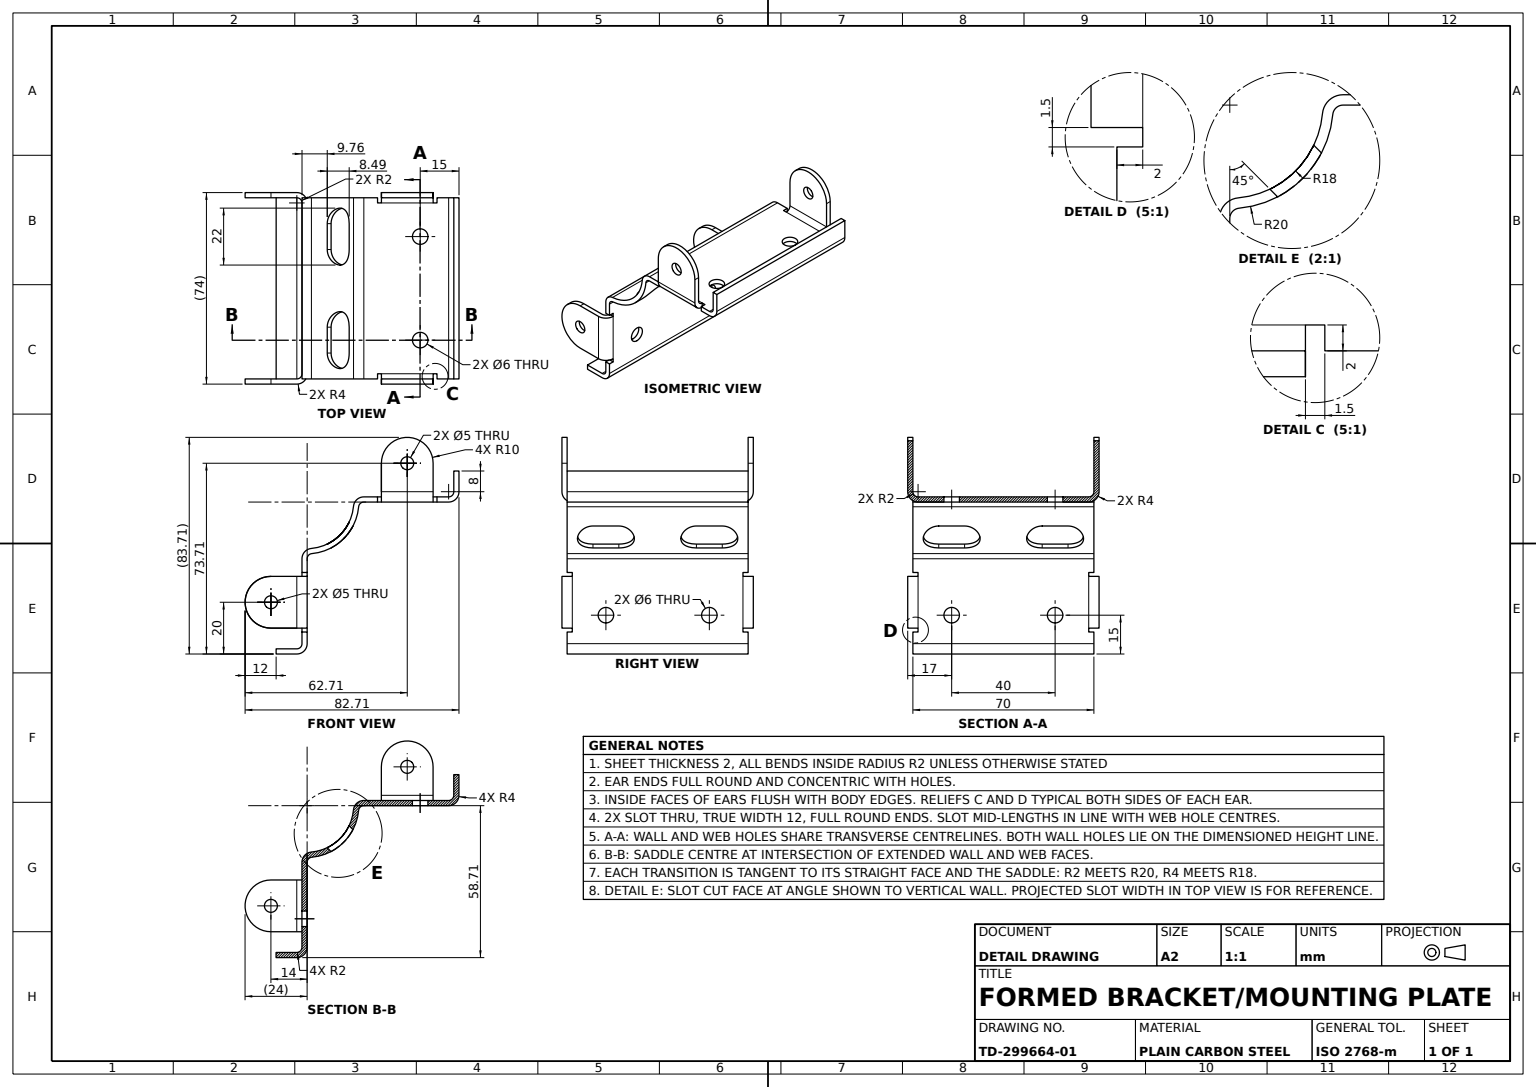
SolidWorks part; units mm, degrees
material "Plain Carbon Steel"
ref_plane "Front Plane" through (0, 0, 0) normal (0, 0, 1) x (1, 0, 0)
ref_plane "Top Plane" through (0, 0, 0) normal (0, 1, 0) x (1, 0, 0)
ref_plane "Right Plane" through (0, 0, 0) normal (1, 0, 0) x (0, 0, -1)
sketch "Saddle Profile Sketch" plane through (0, 0, 0) normal (0, 0, 1) x (1, 0, 0)
  line L0 (-15.4919, -15.4919) -> (-38.6863, -38.6863)
  line L1 (15.4919, -15.4919) -> (38.6863, -38.6863)
  line L9 (-44.3431, -38.6863) -> (-50, -33.0294)
  line L10 (42.9289, -37.2721) -> (48.5858, -31.6152)
  line L11 (44.3431, -38.6863) -> (50, -33.0294)
  line L12 (-50, -50) -> (-50, -50.1773)
  line L13 (-41.5147, -41.5147) -> (-15.4919, -15.4919)
  line L14 (16.9061, -14.0777) -> (40.1005, -37.2721)
  line L15 (-16.9061, -14.0777) -> (-40.1005, -37.2721)
  line L16 (41.5147, -41.5147) -> (15.4919, -15.4919)
  line L17 (-42.9289, -37.2721) -> (-48.5858, -31.6152)
  line L18 (-50, -33.0294) -> (-48.5858, -31.6152)
  line L19 (50, -33.0294) -> (48.5858, -31.6152)
  arc A0 (-12.7979, -15.3692) -> (12.7979, -15.3692) centre (0, 0) ccw
  arc A1 (38.6863, -38.6863) -> (44.3431, -38.6863) centre (41.5147, -35.8579) ccw
  arc A2 (-44.3431, -38.6863) -> (-38.6863, -38.6863) centre (-41.5147, -35.8579) ccw
  arc A3 (12.7979, -15.3692) -> (15.4919, -15.4919) centre (14.0777, -16.9061) cw
  arc A4 (-12.7979, -15.3692) -> (-15.4919, -15.4919) centre (-14.0777, -16.9061) ccw
  arc A5 (40.1005, -37.2721) -> (42.9289, -37.2721) centre (41.5147, -35.8579) ccw
  arc A6 (11.5181, -13.8323) -> (16.9061, -14.0777) centre (14.0777, -16.9061) cw
  arc A7 (-11.5181, -13.8323) -> (11.5181, -13.8323) centre (0, 0) ccw
  arc A8 (-11.5181, -13.8323) -> (-16.9061, -14.0777) centre (-14.0777, -16.9061) ccw
  arc A9 (-42.9289, -37.2721) -> (-40.1005, -37.2721) centre (-41.5147, -35.8579) ccw
  point P8 (0, 0)
  dimension "D1" = 40
  dimension "D5" = 4
  dimension "D6" = 2
  dimension "D2" = 45
  dimension "D3" = 45
  dimension "D4" = 8.4853
  dimension "D7" = 50
  dimension "D8" = 50
  dimension "D9" = 23.1944
  dimension "D10" = 23.1944
  dimension "D11" = 8
  dimension "D13" = 0.1773
  dimension "D14" = 50
  dimension "D15" = 50
  dimension "D12" = 2
extrude "Saddle Body 70mm" add sketch "Saddle Profile Sketch" along normal blind 70 contours A9 L17 L18 L9 A2 L0 A4 A0 A3 L1 A1 L11 L19 L10 A5 L14 A6 A7 A8 L15
sketch "Flange Notches Sketch" plane through (0, 0, 0) normal (0, 1, 0) x (1, 0, 0)
  line L0 (-6, -10) -> (-6, -20)
  line L1 (6, -10) -> (6, -20)
  line L2 (16.9061, 0) -> (40.1005, 0) construction
  line L3 (-6, -50) -> (-6, -60)
  line L4 (6, -50) -> (6, -60)
  line L6 (16.9061, -70) -> (40.1005, -70) construction
  line L8 (11.5181, -70) -> (11.5181, 0) construction
  arc A0 (6, -10) -> (-6, -10) centre (0, -10) ccw
  arc A1 (-6, -20) -> (6, -20) centre (0, -20) ccw
  arc A2 (6, -50) -> (-6, -50) centre (0, -50) ccw
  arc A3 (-6, -60) -> (6, -60) centre (0, -60) ccw
  point P1 (6, -15)
  point P5 (6, -55)
  dimension "D1" = 10
  dimension "D2" = 6
  dimension "D3" = 15
  dimension "D5" = 6
  dimension "D4" = 10
  dimension "D6" = 15
  dimension "D7" = 10
  dimension "D8" = 11.5181
extrude "Flange Notches" cut sketch "Flange Notches Sketch" against normal blind 70
sketch "Flange Holes A Sketch" plane through (1.4142, 1.4142, 0) normal (0.7071, 0.7071, 0) x (0, 0, -1)
  line L0 (-70, -21.9089) -> (-70, -54.7107) construction
  line L1 (0, -21.9089) -> (0, -54.7107) construction
  line L3 (-70, -58.7107) -> (0, -58.7107) construction
  circle A0 centre (-55, -43.7107) radius 3
  circle A1 centre (-15, -43.7107) radius 3
  dimension "D1" = 6
  dimension "D2" = 6
  dimension "D3" = 15
  dimension "D4" = 15
  dimension "D5" = 40
  dimension "D6" = 15
extrude "Flange Holes A Ø6" cut sketch "Flange Holes A Sketch" against normal blind 70
sketch "Flange Holes B Sketch" plane through (-1.4142, 1.4142, 0) normal (-0.7071, 0.7071, 0) x (0, 0, 1)
  line L0 (70, -21.9089) -> (70, -54.7107) construction
  line L1 (0, -21.9089) -> (0, -54.7107) construction
  line L2 (70, -58.7107) -> (0, -58.7107) construction
  circle A0 centre (15, -43.7107) radius 3
  circle A1 centre (55, -43.7107) radius 3
  dimension "D1" = 6
  dimension "D2" = 6
  dimension "D3" = 15
  dimension "D4" = 15
  dimension "D5" = 40
  dimension "D6" = 15
extrude "Flange Holes B Ø6" cut sketch "Flange Holes B Sketch" against normal blind 70
sketch "Saddle Slot A Sketch" plane through (-1.4142, 1.4142, 0) normal (-0.7071, 0.7071, 0) x (0, 0, 1)
  line L1 (70, -27.2107) -> (68, -27.2107)
  line L2 (70, -28.7107) -> (0, -28.7107)
  line L3 (70, -28.7107) -> (68, -28.7107)
  line L4 (70, -48.7107) -> (68, -48.7107)
  line L5 (70, -50.2107) -> (68, -50.2107)
  line L9 (2, -27.2107) -> (2, -28.7107)
  line L10 (0, -27.2107) -> (0, -28.7107)
  line L12 (68, -27.2107) -> (68, -28.7107)
  line L13 (70, -27.2107) -> (70, -28.7107)
  line L14 (68, -48.7107) -> (68, -50.2107)
  line L15 (68, -21.9089) -> (68, -54.7107) construction
  line L16 (70, -21.9089) -> (70, -54.7107) construction
  line L17 (70, -48.7107) -> (70, -50.2107)
  line L18 (2, -48.7107) -> (2, -50.2107)
  line L19 (0, -48.7107) -> (0, -50.2107)
  line L20 (2, -27.2107) -> (2, -50.2107) construction
  line L21 (2, -27.2107) -> (0, -27.2107)
  line L22 (0, -27.2107) -> (0, -50.2107) construction
  line L23 (2, -28.7107) -> (0, -28.7107)
  line L24 (70, -27.2107) -> (0, -27.2107) construction
  line L25 (2, -48.7107) -> (0, -48.7107)
  line L26 (70, -28.7107) -> (0, -28.7107) construction
  line L27 (2, -50.2107) -> (0, -50.2107)
  line L28 (70, -48.7107) -> (0, -48.7107) construction
  line L30 (70, -50.2107) -> (0, -50.2107) construction
  dimension "D2" = 1.5
  dimension "D3" = 20
  dimension "D4" = 2
  dimension "D1" = 30
extrude "Saddle Slot A" cut sketch "Saddle Slot A Sketch" against normal blind 70
sketch "Saddle Slot B Sketch" plane through (1.4142, 1.4142, 0) normal (0.7071, 0.7071, 0) x (0, 0, -1)
  line L5 (-70, -48.7107) -> (-68, -48.7107)
  line L6 (-70, -28.7107) -> (0, -28.7107)
  line L7 (-70, -28.7107) -> (-68, -28.7107)
  line L12 (-2, -50.2107) -> (-2, -48.7107)
  line L14 (-68, -27.2107) -> (-68, -28.7107)
  line L16 (-70, -27.2107) -> (-68, -27.2107)
  line L17 (-70, -50.2107) -> (-68, -50.2107)
  line L18 (-70, -27.2107) -> (-70, -28.7107)
  line L19 (0, -50.2107) -> (0, -48.7107)
  line L20 (-2, -28.7107) -> (0, -28.7107)
  line L21 (-70, -23.9089) -> (-70, -52.7107) construction
  line L22 (-68, -23.9089) -> (-68, -52.7107) construction
  line L23 (-2, -52.7107) -> (-2, -23.9089) construction
  line L24 (0, -52.7107) -> (0, -23.9089) construction
  line L25 (-2, -27.2107) -> (0, -27.2107)
  line L26 (-70, -28.7107) -> (0, -28.7107) construction
  line L27 (-68, -48.7107) -> (-68, -50.2107)
  line L28 (-70, -27.2107) -> (0, -27.2107) construction
  line L29 (-70, -48.7107) -> (-70, -50.2107)
  line L30 (-2, -28.7107) -> (-2, -27.2107)
  line L31 (0, -28.7107) -> (0, -27.2107)
  line L32 (-2, -50.2107) -> (0, -50.2107)
  line L33 (-2, -48.7107) -> (0, -48.7107)
  line L34 (-70, -50.2107) -> (0, -50.2107) construction
  line L36 (-70, -48.7107) -> (0, -48.7107) construction
  dimension "D1" = 1.5
  dimension "D3" = 20
  dimension "D4" = 2
  dimension "D2" = 30
extrude "Saddle Slot B" cut sketch "Saddle Slot B Sketch" against normal blind 70
sketch "Mounting Ears A Sketch" plane through (0, 0, 70) normal (0, 0, 1) x (1, 0, 0)
  line L0 (44.3431, -38.6863) -> (50, -33.0294) construction
  line L1 (35.5043, -35.5043) -> (38.6863, -38.6863) construction
  line L2 (34.4437, -34.4437) -> (45.0503, -23.837)
  line L3 (20.3015, -20.3015) -> (34.4437, -34.4437)
  line L4 (-20.3015, -20.3015) -> (-30.201, -10.402)
  line L5 (-20.3015, -20.3015) -> (-34.4437, -34.4437)
  line L6 (-34.4437, -34.4437) -> (-44.3431, -24.5442)
  line L7 (-44.3431, -38.6863) -> (-50, -33.0294) construction
  line L8 (-15.4919, -15.4919) -> (-19.2409, -19.2409) construction
  line L10 (20.3015, -20.3015) -> (30.9081, -9.6949)
  circle A0 centre (37.9792, -16.766) radius 10
  circle A1 centre (37.9792, -16.766) radius 2.5
  circle A2 centre (-37.2721, -17.4731) radius 10
  circle A3 centre (-37.2721, -17.4731) radius 2.5
  line M4 (21.7157, -18.8873) -> (20.3015, -20.3015)
  line M5 (20.3015, -20.3015) -> (34.4437, -34.4437)
  line M6 (34.4437, -34.4437) -> (35.8579, -33.0294)
  line M7 (35.8579, -33.0294) -> (21.7157, -18.8873)
  dimension "D1" = 20
  dimension "D2" = 20
  dimension "D3" = 5
  dimension "D4" = 20
  dimension "D5" = 20
  dimension "D8" = 5
  dimension "D6" = 14
  dimension "D7" = 15
extrude "Mounting Ears A" add sketch "Mounting Ears A Sketch" along normal blind 2 contours A2 A3 | A2 L6 L5 L4 | A0 L10 L2 M7 | A0 A1 | M7 M4 M5 M6
sketch "Mounting Ears B Sketch" plane through (0, 0, 0) normal (0, 0, -1) x (-1, 0, 0)
  line L0 (-30.9081, -9.6949) -> (-20.3015, -20.3015)
  line L1 (-20.3015, -20.3015) -> (-34.4437, -34.4437)
  line L2 (-34.4437, -34.4437) -> (-45.0503, -23.837)
  line L3 (30.201, -10.402) -> (20.3015, -20.3015)
  line L4 (20.3015, -20.3015) -> (34.4437, -34.4437)
  line L5 (34.4437, -34.4437) -> (44.3431, -24.5442)
  arc A0 (-30.9081, -9.6949) -> (-45.0503, -23.837) centre (-37.9792, -16.766) ccw
  circle A1 centre (-37.9792, -16.766) radius 2.5
  circle A2 centre (37.2721, -17.4731) radius 2.5
  arc A3 (44.3431, -24.5442) -> (30.201, -10.402) centre (37.2721, -17.4731) ccw
  dimension "D1" = 5
  dimension "D2" = 5
extrude "Mounting Ears B" add sketch "Mounting Ears B Sketch" along normal blind 2
fillet "Ear Fillets R4" radius 4 4 edges at (27.3726, -27.3726, -2) (27.3726, -27.3726, 72) (-27.3726, -27.3726, 72) (-27.3726, -27.3726, -2)
fillet "Ear Root Fillets R2" radius 2 4 edges at (28.7868, -25.9584, 70) (-28.7868, -25.9584, 70) (28.7868, -25.9584, 0) (-28.7868, -25.9584, 0)
